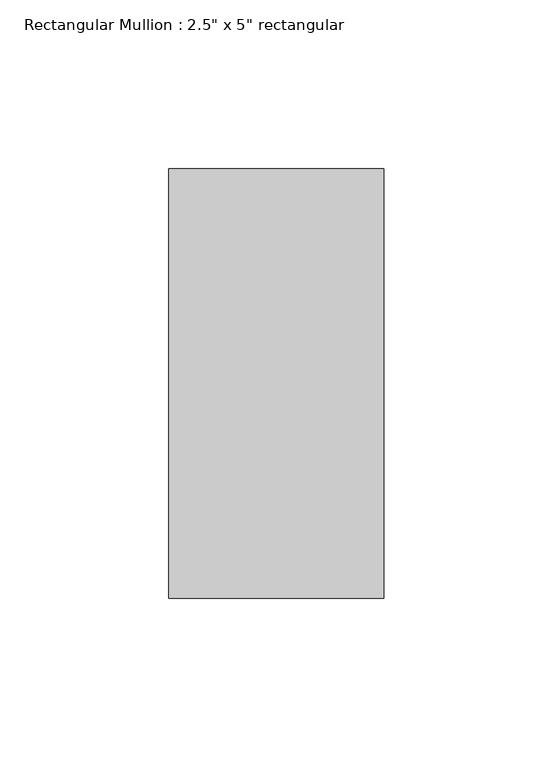
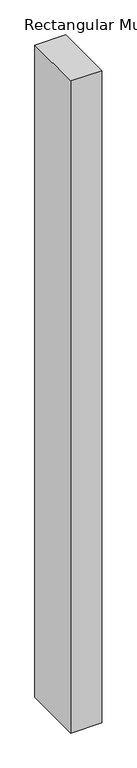
"""IFC4 building model written with IfcOpenShell, lengths in millimetres: member geometry."""

from ifc_helpers import new_model, si_unit, frame, origin, place, context, project, spatial, polyline, outline, extrude, source, transform, mapped, element, save


def member_7022ac76(model_context):
    return source(origin(), model_context, "Body", "SweptSolid", [
        extrude(outline(polyline([(31.75, 63.5), (31.75, -63.5), (-31.75, -63.5), (-31.75, 63.5), (31.75, 63.5)])), frame((0.0, 0.0, -1409.7), z_axis=(0.0, 0.0, 1.0), x_axis=(1.0, 0.0, 0.0)), (0.0, 0.0, 1.0), 1409.7),
    ])


if __name__ == "__main__":
    model = new_model("IFC4")
    model_context = context("Model", 3, world=origin())
    ifc_project = project(units=[si_unit("LENGTHUNIT", "METRE", prefix="MILLI")], contexts=[model_context])
    site = spatial("IfcSite", under=ifc_project)
    building = spatial("IfcBuilding", under=site)
    placement = place(None, origin())
    member_shape = member_7022ac76(model_context)
    element("IfcMember", 1, ObjectType="Rectangular Mullion : 2.5\" x 5\" rectangular", at=placement, inside=building, context=model_context, shape_type="MappedRepresentation", body=[
        mapped(member_shape, transform((0.0, 0.0, 0.0), x_axis=(1.0, 0.0, 0.0), y_axis=(0.0, 1.0, 0.0), z_axis=(0.0, 0.0, 1.0))),
    ])
    save(model, "model.ifc")

# Revit data of these elements
# Type "Rectangular Mullion : 2.5\" x 5\" rectangular"
#   built-in parameter 1007304 = 0.416667 (stored number, unit not read)
#   built-in parameter 1007301 = 0.104167 (stored number, unit not read)
#   built-in parameter 1007300 = 0.104167 (stored number, unit not read)
# Element 1 (IfcMember, "Rectangular Mullion : 2.5\" x 5\" rectangular")
#   Materials on its faces: "Aluminum"
# Materials
#   "Aluminum": class "Metal", colour RGB 247 247 247, transparency 0, Description = "Aluminum 6061", Cost = 0
